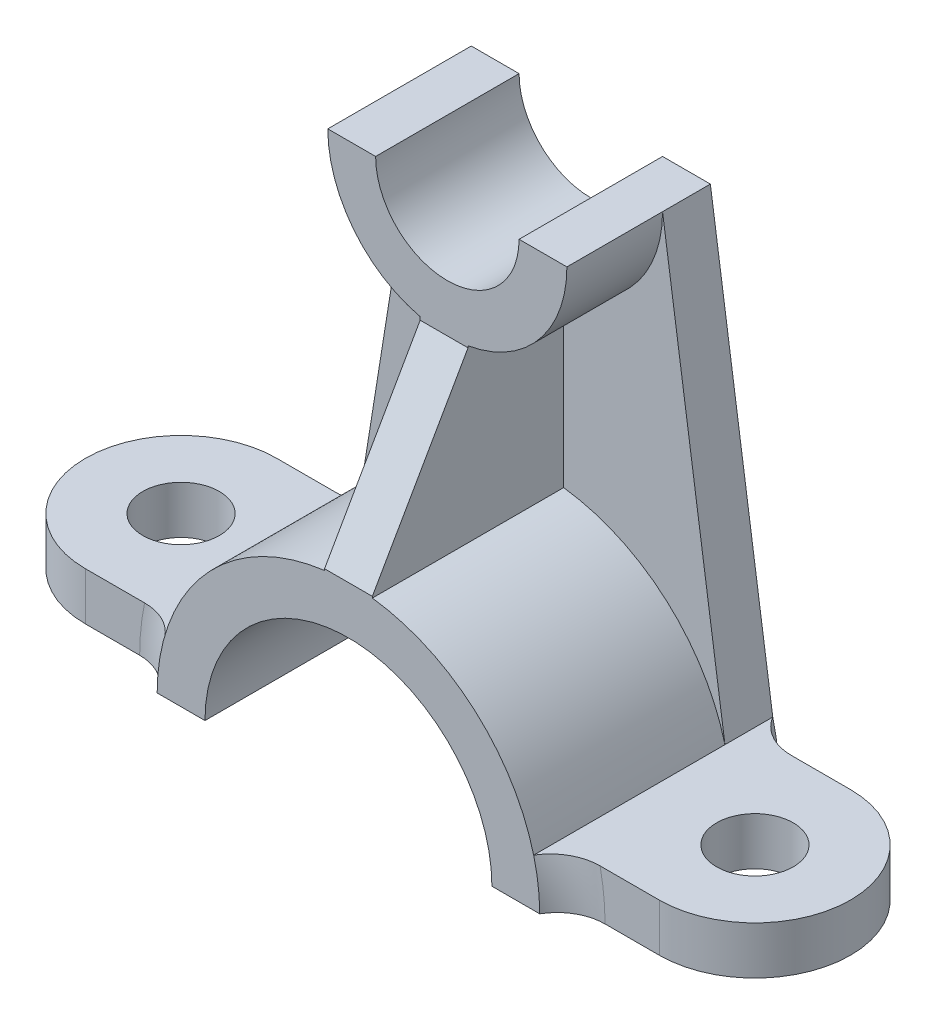
ISO-10303-21;
HEADER;
FILE_DESCRIPTION(('STEP AP214'),'2;1');
FILE_NAME('part.step','',(''),(''),'','','');
FILE_SCHEMA(('AUTOMOTIVE_DESIGN { 1 0 10303 214 1 1 1 1 }'));
ENDSEC;
DATA;
#1=APPLICATION_CONTEXT('core data for automotive mechanical design processes');
#2=APPLICATION_PROTOCOL_DEFINITION('international standard','automotive_design',2000,#1);
#3=PRODUCT_CONTEXT('',#1,'mechanical');
#4=PRODUCT('Part','Part','',(#3));
#5=PRODUCT_RELATED_PRODUCT_CATEGORY('part','',(#4));
#6=PRODUCT_DEFINITION_FORMATION('','',#4);
#7=PRODUCT_DEFINITION_CONTEXT('part definition',#1,'design');
#8=PRODUCT_DEFINITION('design','',#6,#7);
#9=PRODUCT_DEFINITION_SHAPE('','',#8);
#10=(LENGTH_UNIT() NAMED_UNIT(*) SI_UNIT(.MILLI.,.METRE.));
#11=(NAMED_UNIT(*) PLANE_ANGLE_UNIT() SI_UNIT($,.RADIAN.));
#12=(NAMED_UNIT(*) SI_UNIT($,.STERADIAN.) SOLID_ANGLE_UNIT());
#13=UNCERTAINTY_MEASURE_WITH_UNIT(LENGTH_MEASURE(1.E-05),#10,'distance_accuracy_value','');
#14=(GEOMETRIC_REPRESENTATION_CONTEXT(3) GLOBAL_UNCERTAINTY_ASSIGNED_CONTEXT((#13)) GLOBAL_UNIT_ASSIGNED_CONTEXT((#10,
#11,#12)) REPRESENTATION_CONTEXT('',''));
#15=CARTESIAN_POINT('',(0.,0.,0.));
#16=DIRECTION('',(0.,0.,1.));
#17=DIRECTION('',(1.,0.,0.));
#18=AXIS2_PLACEMENT_3D('',#15,#16,#17);
#19=CARTESIAN_POINT('',(0.,0.,25.));
#20=DIRECTION('',(0.,0.,-1.));
#21=DIRECTION('',(-1.,0.,0.));
#22=AXIS2_PLACEMENT_3D('',#19,#20,#21);
#23=CYLINDRICAL_SURFACE('',#22,40.);
#24=DIRECTION('',(0.,0.,-1.));
#25=VECTOR('',#24,1.);
#26=CARTESIAN_POINT('',(-5.,39.6862696659689,25.));
#27=LINE('',#26,#25);
#28=CARTESIAN_POINT('',(-5.,39.6862696659689,-15.));
#29=VERTEX_POINT('',#28);
#30=CARTESIAN_POINT('',(-5.,39.6862696659689,25.));
#31=VERTEX_POINT('',#30);
#32=EDGE_CURVE('E251',#29,#31,#27,.F.);
#33=ORIENTED_EDGE('',*,*,#32,.F.);
#34=CARTESIAN_POINT('',(0.,0.,-15.));
#35=DIRECTION('',(0.,0.,1.));
#36=DIRECTION('',(-1.,0.,0.));
#37=AXIS2_PLACEMENT_3D('',#34,#35,#36);
#38=CIRCLE('',#37,40.);
#39=CARTESIAN_POINT('',(-38.7298334620742,10.,-15.));
#40=VERTEX_POINT('',#39);
#41=EDGE_CURVE('E296',#29,#40,#38,.T.);
#42=ORIENTED_EDGE('',*,*,#41,.T.);
#43=DIRECTION('',(0.,0.,-1.));
#44=VECTOR('',#43,1.);
#45=CARTESIAN_POINT('',(-38.7298334620742,10.,25.));
#46=LINE('',#45,#44);
#47=CARTESIAN_POINT('',(-38.7298334620742,10.,25.));
#48=VERTEX_POINT('',#47);
#49=EDGE_CURVE('E399',#40,#48,#46,.F.);
#50=ORIENTED_EDGE('',*,*,#49,.T.);
#51=CARTESIAN_POINT('',(0.,0.,25.));
#52=DIRECTION('',(0.,0.,1.));
#53=DIRECTION('',(1.,0.,0.));
#54=AXIS2_PLACEMENT_3D('',#51,#52,#53);
#55=CIRCLE('',#54,40.);
#56=EDGE_CURVE('E372',#31,#48,#55,.T.);
#57=ORIENTED_EDGE('',*,*,#56,.F.);
#58=EDGE_LOOP('',(#33,#42,#50,#57));
#59=FACE_BOUND('',#58,.T.);
#60=ADVANCED_FACE('F39',(#59),#23,.T.);
#61=CARTESIAN_POINT('',(0.681025672357616,100.,-15.));
#62=DIRECTION('',(0.,0.,-1.));
#63=DIRECTION('',(-1.,0.,0.));
#64=AXIS2_PLACEMENT_3D('',#61,#62,#63);
#65=PLANE('',#64);
#66=DIRECTION('',(0.,-1.,0.));
#67=VECTOR('',#66,1.);
#68=CARTESIAN_POINT('',(-5.,100.,-15.));
#69=LINE('',#68,#67);
#70=CARTESIAN_POINT('',(-5.,75.6540363240636,-15.));
#71=VERTEX_POINT('',#70);
#72=EDGE_CURVE('E253',#71,#29,#69,.T.);
#73=ORIENTED_EDGE('',*,*,#72,.F.);
#74=CARTESIAN_POINT('',(0.681025672357616,100.,-15.));
#75=DIRECTION('',(0.,0.,1.));
#76=DIRECTION('',(-1.,0.,0.));
#77=AXIS2_PLACEMENT_3D('',#74,#75,#76);
#78=CIRCLE('',#77,25.);
#79=CARTESIAN_POINT('',(-24.3189743276424,100.,-15.));
#80=VERTEX_POINT('',#79);
#81=EDGE_CURVE('E291',#80,#71,#78,.T.);
#82=ORIENTED_EDGE('',*,*,#81,.F.);
#83=DIRECTION('',(0.158106665603804,0.987422038589198,0.));
#84=VECTOR('',#83,1.);
#85=CARTESIAN_POINT('',(-24.3189743276424,100.,-15.));
#86=LINE('',#85,#84);
#87=EDGE_CURVE('E303',#40,#80,#86,.T.);
#88=ORIENTED_EDGE('',*,*,#87,.F.);
#89=ORIENTED_EDGE('',*,*,#41,.F.);
#90=EDGE_LOOP('',(#73,#82,#88,#89));
#91=FACE_BOUND('',#90,.T.);
#92=ADVANCED_FACE('F475',(#91),#65,.F.);
#93=CARTESIAN_POINT('',(0.681025672357616,100.,5.));
#94=DIRECTION('',(0.,0.,-1.));
#95=DIRECTION('',(-1.,0.,0.));
#96=AXIS2_PLACEMENT_3D('',#93,#94,#95);
#97=CYLINDRICAL_SURFACE('',#96,25.);
#98=DIRECTION('',(0.,0.,-1.));
#99=VECTOR('',#98,1.);
#100=CARTESIAN_POINT('',(-5.,75.6540363240636,5.));
#101=LINE('',#100,#99);
#102=CARTESIAN_POINT('',(-5.,75.6540363240636,5.));
#103=VERTEX_POINT('',#102);
#104=EDGE_CURVE('E247',#103,#71,#101,.T.);
#105=ORIENTED_EDGE('',*,*,#104,.F.);
#106=CARTESIAN_POINT('',(0.681025672357616,100.,5.));
#107=DIRECTION('',(0.,0.,1.));
#108=DIRECTION('',(1.,0.,0.));
#109=AXIS2_PLACEMENT_3D('',#106,#107,#108);
#110=CIRCLE('',#109,25.);
#111=CARTESIAN_POINT('',(-24.3189743276424,100.,5.));
#112=VERTEX_POINT('',#111);
#113=EDGE_CURVE('E277',#112,#103,#110,.T.);
#114=ORIENTED_EDGE('',*,*,#113,.F.);
#115=DIRECTION('',(0.,0.,-1.));
#116=VECTOR('',#115,1.);
#117=CARTESIAN_POINT('',(-24.3189743276424,100.,5.));
#118=LINE('',#117,#116);
#119=EDGE_CURVE('E286',#112,#80,#118,.T.);
#120=ORIENTED_EDGE('',*,*,#119,.T.);
#121=ORIENTED_EDGE('',*,*,#81,.T.);
#122=EDGE_LOOP('',(#105,#114,#120,#121));
#123=FACE_BOUND('',#122,.T.);
#124=ADVANCED_FACE('F481',(#123),#97,.T.);
#125=CARTESIAN_POINT('',(38.7298334620742,10.,-15.));
#126=VERTEX_POINT('',#125);
#127=CARTESIAN_POINT('',(5.,39.6862696659689,-15.));
#128=VERTEX_POINT('',#127);
#129=EDGE_CURVE('E301',#126,#128,#38,.T.);
#130=ORIENTED_EDGE('',*,*,#129,.T.);
#131=DIRECTION('',(0.,0.,-1.));
#132=VECTOR('',#131,1.);
#133=CARTESIAN_POINT('',(5.,39.6862696659689,25.));
#134=LINE('',#133,#132);
#135=CARTESIAN_POINT('',(5.,39.6862696659689,25.));
#136=VERTEX_POINT('',#135);
#137=EDGE_CURVE('E261',#128,#136,#134,.F.);
#138=ORIENTED_EDGE('',*,*,#137,.T.);
#139=CARTESIAN_POINT('',(38.7298334620742,10.,25.));
#140=VERTEX_POINT('',#139);
#141=EDGE_CURVE('E234',#140,#136,#55,.T.);
#142=ORIENTED_EDGE('',*,*,#141,.F.);
#143=DIRECTION('',(0.,0.,-1.));
#144=VECTOR('',#143,1.);
#145=CARTESIAN_POINT('',(38.7298334620742,10.,25.));
#146=LINE('',#145,#144);
#147=EDGE_CURVE('E68',#126,#140,#146,.F.);
#148=ORIENTED_EDGE('',*,*,#147,.F.);
#149=EDGE_LOOP('',(#130,#138,#142,#148));
#150=FACE_BOUND('',#149,.T.);
#151=ADVANCED_FACE('F478',(#150),#23,.T.);
#152=CARTESIAN_POINT('',(-40.,0.,25.));
#153=DIRECTION('',(0.,1.,0.));
#154=DIRECTION('',(0.,0.,1.));
#155=AXIS2_PLACEMENT_3D('',#152,#153,#154);
#156=PLANE('',#155);
#157=CARTESIAN_POINT('',(-60.,0.,0.));
#158=DIRECTION('',(0.,1.,0.));
#159=DIRECTION('',(0.,0.,1.));
#160=AXIS2_PLACEMENT_3D('',#157,#158,#159);
#161=CIRCLE('',#160,8.);
#162=CARTESIAN_POINT('',(-60.,0.,8.));
#163=VERTEX_POINT('',#162);
#164=EDGE_CURVE('E314',#163,#163,#161,.T.);
#165=ORIENTED_EDGE('',*,*,#164,.T.);
#166=EDGE_LOOP('',(#165));
#167=FACE_BOUND('',#166,.T.);
#168=DIRECTION('',(1.,0.,0.));
#169=VECTOR('',#168,1.);
#170=CARTESIAN_POINT('',(-40.,0.,25.));
#171=LINE('',#170,#169);
#172=CARTESIAN_POINT('',(-40.,0.,25.));
#173=VERTEX_POINT('',#172);
#174=CARTESIAN_POINT('',(-30.,0.,25.));
#175=VERTEX_POINT('',#174);
#176=EDGE_CURVE('E373',#173,#175,#171,.T.);
#177=ORIENTED_EDGE('',*,*,#176,.F.);
#178=CARTESIAN_POINT('',(-48.6602540378444,0.,30.));
#179=DIRECTION('',(0.,1.,0.));
#180=DIRECTION('',(0.,0.,1.));
#181=AXIS2_PLACEMENT_3D('',#178,#179,#180);
#182=CIRCLE('',#181,10.);
#183=CARTESIAN_POINT('',(-48.6602540378444,0.,20.));
#184=VERTEX_POINT('',#183);
#185=EDGE_CURVE('E52',#173,#184,#182,.T.);
#186=ORIENTED_EDGE('',*,*,#185,.T.);
#187=DIRECTION('',(-1.,0.,0.));
#188=VECTOR('',#187,1.);
#189=CARTESIAN_POINT('',(-35.,0.,20.));
#190=LINE('',#189,#188);
#191=CARTESIAN_POINT('',(-60.,0.,20.));
#192=VERTEX_POINT('',#191);
#193=EDGE_CURVE('E341',#184,#192,#190,.T.);
#194=ORIENTED_EDGE('',*,*,#193,.T.);
#195=CARTESIAN_POINT('',(-60.,0.,0.));
#196=DIRECTION('',(0.,-1.,0.));
#197=DIRECTION('',(0.,0.,1.));
#198=AXIS2_PLACEMENT_3D('',#195,#196,#197);
#199=CIRCLE('',#198,20.);
#200=CARTESIAN_POINT('',(-60.,0.,-20.));
#201=VERTEX_POINT('',#200);
#202=EDGE_CURVE('E340',#192,#201,#199,.T.);
#203=ORIENTED_EDGE('',*,*,#202,.T.);
#204=DIRECTION('',(1.,0.,0.));
#205=VECTOR('',#204,1.);
#206=CARTESIAN_POINT('',(-35.,0.,-20.));
#207=LINE('',#206,#205);
#208=CARTESIAN_POINT('',(-48.6602540378444,0.,-20.));
#209=VERTEX_POINT('',#208);
#210=EDGE_CURVE('E331',#201,#209,#207,.T.);
#211=ORIENTED_EDGE('',*,*,#210,.T.);
#212=CARTESIAN_POINT('',(-48.6602540378444,0.,-30.));
#213=DIRECTION('',(0.,1.,0.));
#214=DIRECTION('',(0.,0.,1.));
#215=AXIS2_PLACEMENT_3D('',#212,#213,#214);
#216=CIRCLE('',#215,10.);
#217=CARTESIAN_POINT('',(-40.,0.,-25.));
#218=VERTEX_POINT('',#217);
#219=EDGE_CURVE('E420',#209,#218,#216,.T.);
#220=ORIENTED_EDGE('',*,*,#219,.T.);
#221=DIRECTION('',(1.,0.,0.));
#222=VECTOR('',#221,1.);
#223=CARTESIAN_POINT('',(-40.,0.,-25.));
#224=LINE('',#223,#222);
#225=CARTESIAN_POINT('',(-30.,0.,-25.));
#226=VERTEX_POINT('',#225);
#227=EDGE_CURVE('E384',#218,#226,#224,.T.);
#228=ORIENTED_EDGE('',*,*,#227,.T.);
#229=DIRECTION('',(0.,0.,-1.));
#230=VECTOR('',#229,1.);
#231=CARTESIAN_POINT('',(-30.,0.,25.));
#232=LINE('',#231,#230);
#233=EDGE_CURVE('E391',#175,#226,#232,.T.);
#234=ORIENTED_EDGE('',*,*,#233,.F.);
#235=EDGE_LOOP('',(#177,#186,#194,#203,#211,#220,#228,#234));
#236=FACE_BOUND('',#235,.T.);
#237=ADVANCED_FACE('F488',(#167,#236),#156,.F.);
#238=CARTESIAN_POINT('',(0.,0.,25.));
#239=DIRECTION('',(0.,0.,-1.));
#240=DIRECTION('',(-1.,0.,0.));
#241=AXIS2_PLACEMENT_3D('',#238,#239,#240);
#242=CYLINDRICAL_SURFACE('',#241,30.);
#243=DIRECTION('',(0.,0.,-1.));
#244=VECTOR('',#243,1.);
#245=CARTESIAN_POINT('',(30.,0.,25.));
#246=LINE('',#245,#244);
#247=CARTESIAN_POINT('',(30.,0.,25.));
#248=VERTEX_POINT('',#247);
#249=CARTESIAN_POINT('',(30.,0.,-25.));
#250=VERTEX_POINT('',#249);
#251=EDGE_CURVE('E381',#248,#250,#246,.T.);
#252=ORIENTED_EDGE('',*,*,#251,.F.);
#253=CARTESIAN_POINT('',(0.,0.,25.));
#254=DIRECTION('',(0.,0.,-1.));
#255=DIRECTION('',(1.,0.,0.));
#256=AXIS2_PLACEMENT_3D('',#253,#254,#255);
#257=CIRCLE('',#256,30.);
#258=EDGE_CURVE('E376',#175,#248,#257,.T.);
#259=ORIENTED_EDGE('',*,*,#258,.F.);
#260=ORIENTED_EDGE('',*,*,#233,.T.);
#261=CARTESIAN_POINT('',(0.,0.,-25.));
#262=DIRECTION('',(0.,0.,-1.));
#263=DIRECTION('',(1.,0.,0.));
#264=AXIS2_PLACEMENT_3D('',#261,#262,#263);
#265=CIRCLE('',#264,30.);
#266=EDGE_CURVE('E390',#226,#250,#265,.T.);
#267=ORIENTED_EDGE('',*,*,#266,.T.);
#268=EDGE_LOOP('',(#252,#259,#260,#267));
#269=FACE_BOUND('',#268,.T.);
#270=ADVANCED_FACE('F493',(#269),#242,.F.);
#271=CARTESIAN_POINT('',(30.,0.,25.));
#272=DIRECTION('',(0.,1.,0.));
#273=DIRECTION('',(0.,0.,1.));
#274=AXIS2_PLACEMENT_3D('',#271,#272,#273);
#275=PLANE('',#274);
#276=CARTESIAN_POINT('',(60.,0.,0.));
#277=DIRECTION('',(0.,1.,0.));
#278=DIRECTION('',(0.,0.,1.));
#279=AXIS2_PLACEMENT_3D('',#276,#277,#278);
#280=CIRCLE('',#279,8.00000000000001);
#281=CARTESIAN_POINT('',(60.,0.,8.00000000000001));
#282=VERTEX_POINT('',#281);
#283=EDGE_CURVE('E320',#282,#282,#280,.T.);
#284=ORIENTED_EDGE('',*,*,#283,.T.);
#285=EDGE_LOOP('',(#284));
#286=FACE_BOUND('',#285,.T.);
#287=DIRECTION('',(1.,0.,0.));
#288=VECTOR('',#287,1.);
#289=CARTESIAN_POINT('',(30.,0.,-25.));
#290=LINE('',#289,#288);
#291=CARTESIAN_POINT('',(40.,0.,-25.));
#292=VERTEX_POINT('',#291);
#293=EDGE_CURVE('E386',#250,#292,#290,.T.);
#294=ORIENTED_EDGE('',*,*,#293,.T.);
#295=CARTESIAN_POINT('',(48.6602540378444,0.,-30.));
#296=DIRECTION('',(0.,1.,0.));
#297=DIRECTION('',(0.,0.,1.));
#298=AXIS2_PLACEMENT_3D('',#295,#296,#297);
#299=CIRCLE('',#298,10.);
#300=CARTESIAN_POINT('',(48.6602540378444,0.,-20.));
#301=VERTEX_POINT('',#300);
#302=EDGE_CURVE('E576',#292,#301,#299,.T.);
#303=ORIENTED_EDGE('',*,*,#302,.T.);
#304=DIRECTION('',(1.,0.,0.));
#305=VECTOR('',#304,1.);
#306=CARTESIAN_POINT('',(35.,0.,-20.));
#307=LINE('',#306,#305);
#308=CARTESIAN_POINT('',(60.,0.,-20.));
#309=VERTEX_POINT('',#308);
#310=EDGE_CURVE('E343',#301,#309,#307,.T.);
#311=ORIENTED_EDGE('',*,*,#310,.T.);
#312=CARTESIAN_POINT('',(60.,0.,0.));
#313=DIRECTION('',(0.,-1.,0.));
#314=DIRECTION('',(0.,0.,-1.));
#315=AXIS2_PLACEMENT_3D('',#312,#313,#314);
#316=CIRCLE('',#315,20.);
#317=CARTESIAN_POINT('',(60.,0.,20.));
#318=VERTEX_POINT('',#317);
#319=EDGE_CURVE('E363',#309,#318,#316,.T.);
#320=ORIENTED_EDGE('',*,*,#319,.T.);
#321=DIRECTION('',(-1.,0.,0.));
#322=VECTOR('',#321,1.);
#323=CARTESIAN_POINT('',(35.,0.,20.));
#324=LINE('',#323,#322);
#325=CARTESIAN_POINT('',(48.6602540378444,0.,20.));
#326=VERTEX_POINT('',#325);
#327=EDGE_CURVE('E353',#318,#326,#324,.T.);
#328=ORIENTED_EDGE('',*,*,#327,.T.);
#329=CARTESIAN_POINT('',(48.6602540378444,0.,30.));
#330=DIRECTION('',(0.,1.,0.));
#331=DIRECTION('',(0.,0.,1.));
#332=AXIS2_PLACEMENT_3D('',#329,#330,#331);
#333=CIRCLE('',#332,10.);
#334=CARTESIAN_POINT('',(40.,0.,25.));
#335=VERTEX_POINT('',#334);
#336=EDGE_CURVE('E460',#326,#335,#333,.T.);
#337=ORIENTED_EDGE('',*,*,#336,.T.);
#338=DIRECTION('',(1.,0.,0.));
#339=VECTOR('',#338,1.);
#340=CARTESIAN_POINT('',(30.,0.,25.));
#341=LINE('',#340,#339);
#342=EDGE_CURVE('E378',#248,#335,#341,.T.);
#343=ORIENTED_EDGE('',*,*,#342,.F.);
#344=ORIENTED_EDGE('',*,*,#251,.T.);
#345=EDGE_LOOP('',(#294,#303,#311,#320,#328,#337,#343,#344));
#346=FACE_BOUND('',#345,.T.);
#347=ADVANCED_FACE('F804',(#286,#346),#275,.F.);
#348=CARTESIAN_POINT('',(0.,0.,25.));
#349=DIRECTION('',(0.,0.,1.));
#350=DIRECTION('',(1.,0.,0.));
#351=AXIS2_PLACEMENT_3D('',#348,#349,#350);
#352=PLANE('',#351);
#353=ORIENTED_EDGE('',*,*,#141,.T.);
#354=DIRECTION('',(0.,1.,0.));
#355=VECTOR('',#354,1.);
#356=CARTESIAN_POINT('',(5.,50.,25.));
#357=LINE('',#356,#355);
#358=CARTESIAN_POINT('',(5.,40.,25.));
#359=VERTEX_POINT('',#358);
#360=EDGE_CURVE('E226',#136,#359,#357,.T.);
#361=ORIENTED_EDGE('',*,*,#360,.T.);
#362=DIRECTION('',(1.,0.,0.));
#363=VECTOR('',#362,1.);
#364=CARTESIAN_POINT('',(0.,40.,25.));
#365=LINE('',#364,#363);
#366=CARTESIAN_POINT('',(-5.,40.,25.));
#367=VERTEX_POINT('',#366);
#368=EDGE_CURVE('E219',#367,#359,#365,.T.);
#369=ORIENTED_EDGE('',*,*,#368,.F.);
#370=DIRECTION('',(0.,1.,0.));
#371=VECTOR('',#370,1.);
#372=CARTESIAN_POINT('',(-5.,50.,25.));
#373=LINE('',#372,#371);
#374=EDGE_CURVE('E242',#31,#367,#373,.T.);
#375=ORIENTED_EDGE('',*,*,#374,.F.);
#376=ORIENTED_EDGE('',*,*,#56,.T.);
#377=EDGE_CURVE('E395',#48,#173,#55,.T.);
#378=ORIENTED_EDGE('',*,*,#377,.T.);
#379=ORIENTED_EDGE('',*,*,#176,.T.);
#380=ORIENTED_EDGE('',*,*,#258,.T.);
#381=ORIENTED_EDGE('',*,*,#342,.T.);
#382=EDGE_CURVE('E371',#335,#140,#55,.T.);
#383=ORIENTED_EDGE('',*,*,#382,.T.);
#384=EDGE_LOOP('',(#353,#361,#369,#375,#376,#378,#379,#380,#381,#383));
#385=FACE_BOUND('',#384,.T.);
#386=ADVANCED_FACE('F233',(#385),#352,.T.);
#387=CARTESIAN_POINT('',(0.,0.,-25.));
#388=DIRECTION('',(0.,0.,1.));
#389=DIRECTION('',(1.,0.,0.));
#390=AXIS2_PLACEMENT_3D('',#387,#388,#389);
#391=PLANE('',#390);
#392=ORIENTED_EDGE('',*,*,#293,.F.);
#393=ORIENTED_EDGE('',*,*,#266,.F.);
#394=ORIENTED_EDGE('',*,*,#227,.F.);
#395=CARTESIAN_POINT('',(0.,0.,-25.));
#396=DIRECTION('',(0.,0.,1.));
#397=DIRECTION('',(1.,0.,0.));
#398=AXIS2_PLACEMENT_3D('',#395,#396,#397);
#399=CIRCLE('',#398,40.);
#400=CARTESIAN_POINT('',(-38.7298334620742,10.,-25.));
#401=VERTEX_POINT('',#400);
#402=EDGE_CURVE('E366',#401,#218,#399,.T.);
#403=ORIENTED_EDGE('',*,*,#402,.F.);
#404=DIRECTION('',(0.158106665603804,0.987422038589198,0.));
#405=VECTOR('',#404,1.);
#406=CARTESIAN_POINT('',(-24.3189743276424,100.,-25.));
#407=LINE('',#406,#405);
#408=CARTESIAN_POINT('',(-24.3189743276424,100.,-25.));
#409=VERTEX_POINT('',#408);
#410=EDGE_CURVE('E310',#401,#409,#407,.T.);
#411=ORIENTED_EDGE('',*,*,#410,.T.);
#412=DIRECTION('',(-1.,0.,0.));
#413=VECTOR('',#412,1.);
#414=CARTESIAN_POINT('',(-24.3189743276424,100.,-25.));
#415=LINE('',#414,#413);
#416=CARTESIAN_POINT('',(-14.3189743276424,100.,-25.));
#417=VERTEX_POINT('',#416);
#418=EDGE_CURVE('E264',#417,#409,#415,.T.);
#419=ORIENTED_EDGE('',*,*,#418,.F.);
#420=CARTESIAN_POINT('',(0.681025672357616,100.,-25.));
#421=DIRECTION('',(0.,0.,-1.));
#422=DIRECTION('',(1.,0.,0.));
#423=AXIS2_PLACEMENT_3D('',#420,#421,#422);
#424=CIRCLE('',#423,15.);
#425=CARTESIAN_POINT('',(15.6810256723576,100.,-25.));
#426=VERTEX_POINT('',#425);
#427=EDGE_CURVE('E263',#426,#417,#424,.T.);
#428=ORIENTED_EDGE('',*,*,#427,.F.);
#429=DIRECTION('',(-1.,0.,0.));
#430=VECTOR('',#429,1.);
#431=CARTESIAN_POINT('',(15.6810256723576,100.,-25.));
#432=LINE('',#431,#430);
#433=CARTESIAN_POINT('',(25.6810256723576,100.,-25.));
#434=VERTEX_POINT('',#433);
#435=EDGE_CURVE('E268',#434,#426,#432,.T.);
#436=ORIENTED_EDGE('',*,*,#435,.F.);
#437=DIRECTION('',(0.143486470703755,-0.989652278694381,0.));
#438=VECTOR('',#437,1.);
#439=CARTESIAN_POINT('',(25.6810256723576,100.,-25.));
#440=LINE('',#439,#438);
#441=CARTESIAN_POINT('',(38.7298334620742,10.,-25.));
#442=VERTEX_POINT('',#441);
#443=EDGE_CURVE('E295',#434,#442,#440,.T.);
#444=ORIENTED_EDGE('',*,*,#443,.T.);
#445=EDGE_CURVE('E385',#292,#442,#399,.T.);
#446=ORIENTED_EDGE('',*,*,#445,.F.);
#447=EDGE_LOOP('',(#392,#393,#394,#403,#411,#419,#428,#436,#444,#446));
#448=FACE_BOUND('',#447,.T.);
#449=ADVANCED_FACE('F439',(#448),#391,.F.);
#450=CARTESIAN_POINT('',(60.,10.,0.));
#451=DIRECTION('',(0.,-1.,0.));
#452=DIRECTION('',(0.,0.,-1.));
#453=AXIS2_PLACEMENT_3D('',#450,#451,#452);
#454=PLANE('',#453);
#455=CARTESIAN_POINT('',(60.,10.,0.));
#456=DIRECTION('',(0.,1.,0.));
#457=DIRECTION('',(0.,0.,1.));
#458=AXIS2_PLACEMENT_3D('',#455,#456,#457);
#459=CIRCLE('',#458,8.00000000000001);
#460=CARTESIAN_POINT('',(60.,10.,8.00000000000001));
#461=VERTEX_POINT('',#460);
#462=EDGE_CURVE('E321',#461,#461,#459,.T.);
#463=ORIENTED_EDGE('',*,*,#462,.F.);
#464=EDGE_LOOP('',(#463));
#465=FACE_BOUND('',#464,.T.);
#466=DIRECTION('',(1.,0.,0.));
#467=VECTOR('',#466,1.);
#468=CARTESIAN_POINT('',(35.,10.,-20.));
#469=LINE('',#468,#467);
#470=CARTESIAN_POINT('',(47.6216371309046,10.,-20.));
#471=VERTEX_POINT('',#470);
#472=CARTESIAN_POINT('',(60.,10.,-20.));
#473=VERTEX_POINT('',#472);
#474=EDGE_CURVE('E348',#471,#473,#469,.T.);
#475=ORIENTED_EDGE('',*,*,#474,.F.);
#476=CARTESIAN_POINT('',(47.6216371309046,10.,-20.));
#477=CARTESIAN_POINT('',(47.3275635647128,10.,-19.9999725811996));
#478=CARTESIAN_POINT('',(47.0334977113731,10.,-20.01242289388));
#479=CARTESIAN_POINT('',(46.4474700390628,10.,-20.0620205132552));
#480=CARTESIAN_POINT('',(46.155508114054,10.,-20.0991665663559));
#481=CARTESIAN_POINT('',(45.575958192143,10.,-20.1978612196002));
#482=CARTESIAN_POINT('',(45.2883671585936,10.,-20.2593919906349));
#483=CARTESIAN_POINT('',(44.7193773078864,10.,-20.4064113995505));
#484=CARTESIAN_POINT('',(44.4379784487489,10.,-20.4918998749561));
#485=CARTESIAN_POINT('',(43.883221966373,10.,-20.686310813259));
#486=CARTESIAN_POINT('',(43.6098688058399,10.,-20.7952460129183));
#487=CARTESIAN_POINT('',(43.0732082863903,10.,-21.0358552040146));
#488=CARTESIAN_POINT('',(42.809905561898,10.,-21.1675395344293));
#489=CARTESIAN_POINT('',(42.295507191387,10.,-21.4526919145932));
#490=CARTESIAN_POINT('',(42.0444066771186,10.,-21.6061511795191));
#491=CARTESIAN_POINT('',(41.5562899807496,10.,-21.9338095330143));
#492=CARTESIAN_POINT('',(41.319267310127,10.,-22.1079989540299));
#493=CARTESIAN_POINT('',(40.8558274604119,10.,-22.4801785915545));
#494=CARTESIAN_POINT('',(40.6297696026495,10.,-22.6786166712502));
#495=CARTESIAN_POINT('',(40.1960204197636,10.,-23.0946419762966));
#496=CARTESIAN_POINT('',(39.9883288915656,10.,-23.3122289898663));
#497=CARTESIAN_POINT('',(39.5925441910588,10.,-23.7656411050683));
#498=CARTESIAN_POINT('',(39.4045075329251,10.,-24.0015155760535));
#499=CARTESIAN_POINT('',(39.0503222140867,10.,-24.4892347345405));
#500=CARTESIAN_POINT('',(38.8841782881545,10.,-24.7410828592982));
#501=CARTESIAN_POINT('',(38.7298334620742,10.,-25.));
#502=B_SPLINE_CURVE_WITH_KNOTS('',3,(#476,#477,#478,#479,#480,#481,#482,#483,#484,#485,#486,
#487,#488,#489,#490,#491,#492,#493,#494,#495,#496,#497,#498,#499,#500,#501),.UNSPECIFIED.,.F.,
.F.,(4,2,2,2,2,2,2,2,2,2,2,2,4),(0.,0.881946521958427,1.76384827836067,2.64510641038706,
3.52635856607926,4.40809065046293,5.2902245219269,6.17200351413211,7.05337288641838,
7.95460227176324,8.85582169106561,9.75956497952399,10.6635034021589),.UNSPECIFIED.);
#503=EDGE_CURVE('E443',#471,#442,#502,.T.);
#504=ORIENTED_EDGE('',*,*,#503,.T.);
#505=EDGE_CURVE('E398',#442,#126,#146,.F.);
#506=ORIENTED_EDGE('',*,*,#505,.T.);
#507=ORIENTED_EDGE('',*,*,#147,.T.);
#508=CARTESIAN_POINT('',(38.7298334620742,10.,25.));
#509=CARTESIAN_POINT('',(38.8768130946296,10.,24.7534474368264));
#510=CARTESIAN_POINT('',(39.0344881880788,10.,24.5132998701854));
#511=CARTESIAN_POINT('',(39.3697661682135,10.,24.0474146522238));
#512=CARTESIAN_POINT('',(39.5473649268116,10.,23.821674031005));
#513=CARTESIAN_POINT('',(39.9206019875073,10.,23.3866670743957));
#514=CARTESIAN_POINT('',(40.1161920586549,10.,23.1773593289555));
#515=CARTESIAN_POINT('',(40.5242729292274,10.,22.7759168816667));
#516=CARTESIAN_POINT('',(40.7367642892412,10.,22.5837827498889));
#517=CARTESIAN_POINT('',(41.1769775394081,10.,22.2179742792945));
#518=CARTESIAN_POINT('',(41.4046951784532,10.,22.0442948227889));
#519=CARTESIAN_POINT('',(41.8738510913466,10.,21.7163510300474));
#520=CARTESIAN_POINT('',(42.1152953822557,10.,21.5620953049238));
#521=CARTESIAN_POINT('',(42.6102602764297,10.,21.2739519840888));
#522=CARTESIAN_POINT('',(42.8637887877046,10.,21.1400779734591));
#523=CARTESIAN_POINT('',(43.380892368368,10.,20.8937049439873));
#524=CARTESIAN_POINT('',(43.6444633858867,10.,20.7811974117538));
#525=CARTESIAN_POINT('',(44.2074399218215,10.,20.5677750708857));
#526=CARTESIAN_POINT('',(44.507748060584,10.,20.4692329711595));
#527=CARTESIAN_POINT('',(45.1160624466181,10.,20.2996699213064));
#528=CARTESIAN_POINT('',(45.4240695595761,10.,20.2286520810099));
#529=CARTESIAN_POINT('',(46.0457021235101,10.,20.1146504402653));
#530=CARTESIAN_POINT('',(46.3593351985563,10.,20.0717081872946));
#531=CARTESIAN_POINT('',(46.9891881697605,10.,20.0143649506646));
#532=CARTESIAN_POINT('',(47.3054079836948,10.,19.9999630633169));
#533=CARTESIAN_POINT('',(47.6216371309046,10.,20.));
#534=B_SPLINE_CURVE_WITH_KNOTS('',3,(#508,#509,#510,#511,#512,#513,#514,#515,#516,#517,#518,
#519,#520,#521,#522,#523,#524,#525,#526,#527,#528,#529,#530,#531,#532,#533),.UNSPECIFIED.,.F.,
.F.,(4,2,2,2,2,2,2,2,2,2,2,2,4),(0.,0.860812450935914,1.72144687394709,2.57983785811531,
3.43825732563233,4.29643811907591,5.15499803978743,6.01412773684447,6.87291439544276,
7.81978670139646,8.76676595862135,9.71514344396407,10.663490899854),.UNSPECIFIED.);
#535=CARTESIAN_POINT('',(47.6216371309046,10.,20.));
#536=VERTEX_POINT('',#535);
#537=EDGE_CURVE('E451',#140,#536,#534,.T.);
#538=ORIENTED_EDGE('',*,*,#537,.T.);
#539=DIRECTION('',(-1.,0.,0.));
#540=VECTOR('',#539,1.);
#541=CARTESIAN_POINT('',(35.,10.,20.));
#542=LINE('',#541,#540);
#543=CARTESIAN_POINT('',(60.,10.,20.));
#544=VERTEX_POINT('',#543);
#545=EDGE_CURVE('E356',#544,#536,#542,.T.);
#546=ORIENTED_EDGE('',*,*,#545,.F.);
#547=CARTESIAN_POINT('',(60.,10.,0.));
#548=DIRECTION('',(0.,-1.,0.));
#549=DIRECTION('',(0.,0.,-1.));
#550=AXIS2_PLACEMENT_3D('',#547,#548,#549);
#551=CIRCLE('',#550,20.);
#552=EDGE_CURVE('E355',#473,#544,#551,.T.);
#553=ORIENTED_EDGE('',*,*,#552,.F.);
#554=EDGE_LOOP('',(#475,#504,#506,#507,#538,#546,#553));
#555=FACE_BOUND('',#554,.T.);
#556=ADVANCED_FACE('F432',(#465,#555),#454,.F.);
#557=CARTESIAN_POINT('',(35.,10.,20.));
#558=DIRECTION('',(0.,0.,1.));
#559=DIRECTION('',(1.,0.,0.));
#560=AXIS2_PLACEMENT_3D('',#557,#558,#559);
#561=PLANE('',#560);
#562=ORIENTED_EDGE('',*,*,#545,.T.);
#563=CARTESIAN_POINT('',(0.,0.,20.));
#564=DIRECTION('',(0.,0.,1.));
#565=DIRECTION('',(1.,0.,0.));
#566=AXIS2_PLACEMENT_3D('',#563,#564,#565);
#567=CIRCLE('',#566,48.6602540378444);
#568=EDGE_CURVE('E408',#536,#326,#567,.F.);
#569=ORIENTED_EDGE('',*,*,#568,.T.);
#570=ORIENTED_EDGE('',*,*,#327,.F.);
#571=DIRECTION('',(0.,-1.,0.));
#572=VECTOR('',#571,1.);
#573=CARTESIAN_POINT('',(60.,10.,20.));
#574=LINE('',#573,#572);
#575=EDGE_CURVE('E368',#544,#318,#574,.T.);
#576=ORIENTED_EDGE('',*,*,#575,.F.);
#577=EDGE_LOOP('',(#562,#569,#570,#576));
#578=FACE_BOUND('',#577,.T.);
#579=ADVANCED_FACE('F438',(#578),#561,.T.);
#580=CARTESIAN_POINT('',(35.,10.,-20.));
#581=DIRECTION('',(0.,0.,-1.));
#582=DIRECTION('',(-1.,0.,0.));
#583=AXIS2_PLACEMENT_3D('',#580,#581,#582);
#584=PLANE('',#583);
#585=ORIENTED_EDGE('',*,*,#310,.F.);
#586=CARTESIAN_POINT('',(0.,0.,-20.));
#587=DIRECTION('',(0.,0.,-1.));
#588=DIRECTION('',(-1.,0.,0.));
#589=AXIS2_PLACEMENT_3D('',#586,#587,#588);
#590=CIRCLE('',#589,48.6602540378444);
#591=EDGE_CURVE('E407',#301,#471,#590,.F.);
#592=ORIENTED_EDGE('',*,*,#591,.T.);
#593=ORIENTED_EDGE('',*,*,#474,.T.);
#594=DIRECTION('',(0.,-1.,0.));
#595=VECTOR('',#594,1.);
#596=CARTESIAN_POINT('',(60.,10.,-20.));
#597=LINE('',#596,#595);
#598=EDGE_CURVE('E357',#473,#309,#597,.T.);
#599=ORIENTED_EDGE('',*,*,#598,.T.);
#600=EDGE_LOOP('',(#585,#592,#593,#599));
#601=FACE_BOUND('',#600,.T.);
#602=ADVANCED_FACE('F772',(#601),#584,.T.);
#603=CARTESIAN_POINT('',(60.,10.,0.));
#604=DIRECTION('',(0.,-1.,0.));
#605=DIRECTION('',(0.,0.,-1.));
#606=AXIS2_PLACEMENT_3D('',#603,#604,#605);
#607=CYLINDRICAL_SURFACE('',#606,20.);
#608=ORIENTED_EDGE('',*,*,#319,.F.);
#609=ORIENTED_EDGE('',*,*,#598,.F.);
#610=ORIENTED_EDGE('',*,*,#552,.T.);
#611=ORIENTED_EDGE('',*,*,#575,.T.);
#612=EDGE_LOOP('',(#608,#609,#610,#611));
#613=FACE_BOUND('',#612,.T.);
#614=ADVANCED_FACE('F431',(#613),#607,.T.);
#615=CARTESIAN_POINT('',(-60.,10.,0.));
#616=DIRECTION('',(0.,1.,0.));
#617=DIRECTION('',(0.,0.,1.));
#618=AXIS2_PLACEMENT_3D('',#615,#616,#617);
#619=PLANE('',#618);
#620=CARTESIAN_POINT('',(-60.,10.,0.));
#621=DIRECTION('',(0.,1.,0.));
#622=DIRECTION('',(0.,0.,1.));
#623=AXIS2_PLACEMENT_3D('',#620,#621,#622);
#624=CIRCLE('',#623,8.);
#625=CARTESIAN_POINT('',(-60.,10.,8.));
#626=VERTEX_POINT('',#625);
#627=EDGE_CURVE('E322',#626,#626,#624,.T.);
#628=ORIENTED_EDGE('',*,*,#627,.F.);
#629=EDGE_LOOP('',(#628));
#630=FACE_BOUND('',#629,.T.);
#631=EDGE_CURVE('E402',#401,#40,#46,.F.);
#632=ORIENTED_EDGE('',*,*,#631,.F.);
#633=CARTESIAN_POINT('',(-38.7298334620742,10.,-25.));
#634=CARTESIAN_POINT('',(-38.8768130946296,10.,-24.7534474368264));
#635=CARTESIAN_POINT('',(-39.0344881880788,10.,-24.5132998701854));
#636=CARTESIAN_POINT('',(-39.3697661682135,10.,-24.0474146522238));
#637=CARTESIAN_POINT('',(-39.5473649268116,10.,-23.821674031005));
#638=CARTESIAN_POINT('',(-39.9206019875073,10.,-23.3866670743957));
#639=CARTESIAN_POINT('',(-40.1161920586549,10.,-23.1773593289555));
#640=CARTESIAN_POINT('',(-40.5242729292274,10.,-22.7759168816667));
#641=CARTESIAN_POINT('',(-40.7367642892412,10.,-22.5837827498889));
#642=CARTESIAN_POINT('',(-41.1769775394081,10.,-22.2179742792945));
#643=CARTESIAN_POINT('',(-41.4046951784532,10.,-22.0442948227889));
#644=CARTESIAN_POINT('',(-41.8738510913466,10.,-21.7163510300474));
#645=CARTESIAN_POINT('',(-42.1152953822557,10.,-21.5620953049238));
#646=CARTESIAN_POINT('',(-42.6102602764297,10.,-21.2739519840888));
#647=CARTESIAN_POINT('',(-42.8637887877046,10.,-21.1400779734591));
#648=CARTESIAN_POINT('',(-43.380892368368,10.,-20.8937049439873));
#649=CARTESIAN_POINT('',(-43.6444633858867,10.,-20.7811974117538));
#650=CARTESIAN_POINT('',(-44.2074399218215,10.,-20.5677750708857));
#651=CARTESIAN_POINT('',(-44.507748060584,10.,-20.4692329711595));
#652=CARTESIAN_POINT('',(-45.1160624466181,10.,-20.2996699213064));
#653=CARTESIAN_POINT('',(-45.4240695595761,10.,-20.2286520810099));
#654=CARTESIAN_POINT('',(-46.0457021235101,10.,-20.1146504402653));
#655=CARTESIAN_POINT('',(-46.3593351985563,10.,-20.0717081872946));
#656=CARTESIAN_POINT('',(-46.9891881697605,10.,-20.0143649506646));
#657=CARTESIAN_POINT('',(-47.3054079836948,10.,-19.9999630633169));
#658=CARTESIAN_POINT('',(-47.6216371309046,10.,-20.));
#659=B_SPLINE_CURVE_WITH_KNOTS('',3,(#633,#634,#635,#636,#637,#638,#639,#640,#641,#642,#643,
#644,#645,#646,#647,#648,#649,#650,#651,#652,#653,#654,#655,#656,#657,#658),.UNSPECIFIED.,.F.,
.F.,(4,2,2,2,2,2,2,2,2,2,2,2,4),(0.,0.860812450935914,1.72144687394709,2.57983785811531,
3.43825732563233,4.29643811907591,5.15499803978743,6.01412773684447,6.87291439544276,
7.81978670139646,8.76676595862135,9.71514344396407,10.663490899854),.UNSPECIFIED.);
#660=CARTESIAN_POINT('',(-47.6216371309046,10.,-20.));
#661=VERTEX_POINT('',#660);
#662=EDGE_CURVE('E415',#401,#661,#659,.T.);
#663=ORIENTED_EDGE('',*,*,#662,.T.);
#664=DIRECTION('',(1.,0.,0.));
#665=VECTOR('',#664,1.);
#666=CARTESIAN_POINT('',(-35.,10.,-20.));
#667=LINE('',#666,#665);
#668=CARTESIAN_POINT('',(-60.,10.,-20.));
#669=VERTEX_POINT('',#668);
#670=EDGE_CURVE('E335',#669,#661,#667,.T.);
#671=ORIENTED_EDGE('',*,*,#670,.F.);
#672=CARTESIAN_POINT('',(-60.,10.,0.));
#673=DIRECTION('',(0.,-1.,0.));
#674=DIRECTION('',(0.,0.,1.));
#675=AXIS2_PLACEMENT_3D('',#672,#673,#674);
#676=CIRCLE('',#675,20.);
#677=CARTESIAN_POINT('',(-60.,10.,20.));
#678=VERTEX_POINT('',#677);
#679=EDGE_CURVE('E347',#678,#669,#676,.T.);
#680=ORIENTED_EDGE('',*,*,#679,.F.);
#681=DIRECTION('',(-1.,0.,0.));
#682=VECTOR('',#681,1.);
#683=CARTESIAN_POINT('',(-35.,10.,20.));
#684=LINE('',#683,#682);
#685=CARTESIAN_POINT('',(-47.6216371309046,10.,20.));
#686=VERTEX_POINT('',#685);
#687=EDGE_CURVE('E338',#686,#678,#684,.T.);
#688=ORIENTED_EDGE('',*,*,#687,.F.);
#689=CARTESIAN_POINT('',(-47.6216371309046,10.,20.));
#690=CARTESIAN_POINT('',(-47.3275635647128,10.,19.9999725811996));
#691=CARTESIAN_POINT('',(-47.0334977113731,10.,20.01242289388));
#692=CARTESIAN_POINT('',(-46.4474700390628,10.,20.0620205132552));
#693=CARTESIAN_POINT('',(-46.155508114054,10.,20.0991665663559));
#694=CARTESIAN_POINT('',(-45.575958192143,10.,20.1978612196002));
#695=CARTESIAN_POINT('',(-45.2883671585936,10.,20.2593919906349));
#696=CARTESIAN_POINT('',(-44.7193773078864,10.,20.4064113995505));
#697=CARTESIAN_POINT('',(-44.4379784487489,10.,20.4918998749561));
#698=CARTESIAN_POINT('',(-43.883221966373,10.,20.686310813259));
#699=CARTESIAN_POINT('',(-43.6098688058399,10.,20.7952460129183));
#700=CARTESIAN_POINT('',(-43.0732082863903,10.,21.0358552040146));
#701=CARTESIAN_POINT('',(-42.809905561898,10.,21.1675395344293));
#702=CARTESIAN_POINT('',(-42.295507191387,10.,21.4526919145932));
#703=CARTESIAN_POINT('',(-42.0444066771186,10.,21.6061511795191));
#704=CARTESIAN_POINT('',(-41.5562899807496,10.,21.9338095330143));
#705=CARTESIAN_POINT('',(-41.319267310127,10.,22.1079989540299));
#706=CARTESIAN_POINT('',(-40.8558274604119,10.,22.4801785915545));
#707=CARTESIAN_POINT('',(-40.6297696026495,10.,22.6786166712502));
#708=CARTESIAN_POINT('',(-40.1960204197636,10.,23.0946419762966));
#709=CARTESIAN_POINT('',(-39.9883288915656,10.,23.3122289898663));
#710=CARTESIAN_POINT('',(-39.5925441910588,10.,23.7656411050683));
#711=CARTESIAN_POINT('',(-39.4045075329251,10.,24.0015155760535));
#712=CARTESIAN_POINT('',(-39.0503222140867,10.,24.4892347345405));
#713=CARTESIAN_POINT('',(-38.8841782881545,10.,24.7410828592982));
#714=CARTESIAN_POINT('',(-38.7298334620742,10.,25.));
#715=B_SPLINE_CURVE_WITH_KNOTS('',3,(#689,#690,#691,#692,#693,#694,#695,#696,#697,#698,#699,
#700,#701,#702,#703,#704,#705,#706,#707,#708,#709,#710,#711,#712,#713,#714),.UNSPECIFIED.,.F.,
.F.,(4,2,2,2,2,2,2,2,2,2,2,2,4),(0.,0.881946521958427,1.76384827836067,2.64510641038706,
3.52635856607926,4.40809065046293,5.2902245219269,6.17200351413211,7.05337288641838,
7.95460227176324,8.85582169106561,9.75956497952399,10.6635034021589),.UNSPECIFIED.);
#716=EDGE_CURVE('E11',#686,#48,#715,.T.);
#717=ORIENTED_EDGE('',*,*,#716,.T.);
#718=ORIENTED_EDGE('',*,*,#49,.F.);
#719=EDGE_LOOP('',(#632,#663,#671,#680,#688,#717,#718));
#720=FACE_BOUND('',#719,.T.);
#721=ADVANCED_FACE('F422',(#630,#720),#619,.T.);
#722=CARTESIAN_POINT('',(-35.,10.,-20.));
#723=DIRECTION('',(0.,0.,-1.));
#724=DIRECTION('',(-1.,0.,0.));
#725=AXIS2_PLACEMENT_3D('',#722,#723,#724);
#726=PLANE('',#725);
#727=ORIENTED_EDGE('',*,*,#670,.T.);
#728=CARTESIAN_POINT('',(0.,0.,-20.));
#729=DIRECTION('',(0.,0.,-1.));
#730=DIRECTION('',(-1.,0.,0.));
#731=AXIS2_PLACEMENT_3D('',#728,#729,#730);
#732=CIRCLE('',#731,48.6602540378444);
#733=EDGE_CURVE('E404',#661,#209,#732,.F.);
#734=ORIENTED_EDGE('',*,*,#733,.T.);
#735=ORIENTED_EDGE('',*,*,#210,.F.);
#736=DIRECTION('',(0.,-1.,0.));
#737=VECTOR('',#736,1.);
#738=CARTESIAN_POINT('',(-60.,10.,-20.));
#739=LINE('',#738,#737);
#740=EDGE_CURVE('E319',#669,#201,#739,.T.);
#741=ORIENTED_EDGE('',*,*,#740,.F.);
#742=EDGE_LOOP('',(#727,#734,#735,#741));
#743=FACE_BOUND('',#742,.T.);
#744=ADVANCED_FACE('F429',(#743),#726,.T.);
#745=CARTESIAN_POINT('',(-35.,10.,20.));
#746=DIRECTION('',(0.,0.,1.));
#747=DIRECTION('',(1.,0.,0.));
#748=AXIS2_PLACEMENT_3D('',#745,#746,#747);
#749=PLANE('',#748);
#750=ORIENTED_EDGE('',*,*,#193,.F.);
#751=CARTESIAN_POINT('',(0.,0.,20.));
#752=DIRECTION('',(0.,0.,1.));
#753=DIRECTION('',(1.,0.,0.));
#754=AXIS2_PLACEMENT_3D('',#751,#752,#753);
#755=CIRCLE('',#754,48.6602540378444);
#756=EDGE_CURVE('E406',#184,#686,#755,.F.);
#757=ORIENTED_EDGE('',*,*,#756,.T.);
#758=ORIENTED_EDGE('',*,*,#687,.T.);
#759=DIRECTION('',(0.,-1.,0.));
#760=VECTOR('',#759,1.);
#761=CARTESIAN_POINT('',(-60.,10.,20.));
#762=LINE('',#761,#760);
#763=EDGE_CURVE('E328',#678,#192,#762,.T.);
#764=ORIENTED_EDGE('',*,*,#763,.T.);
#765=EDGE_LOOP('',(#750,#757,#758,#764));
#766=FACE_BOUND('',#765,.T.);
#767=ADVANCED_FACE('F595',(#766),#749,.T.);
#768=CARTESIAN_POINT('',(-60.,10.,0.));
#769=DIRECTION('',(0.,-1.,0.));
#770=DIRECTION('',(0.,0.,-1.));
#771=AXIS2_PLACEMENT_3D('',#768,#769,#770);
#772=CYLINDRICAL_SURFACE('',#771,20.);
#773=ORIENTED_EDGE('',*,*,#202,.F.);
#774=ORIENTED_EDGE('',*,*,#763,.F.);
#775=ORIENTED_EDGE('',*,*,#679,.T.);
#776=ORIENTED_EDGE('',*,*,#740,.T.);
#777=EDGE_LOOP('',(#773,#774,#775,#776));
#778=FACE_BOUND('',#777,.T.);
#779=ADVANCED_FACE('F469',(#778),#772,.T.);
#780=CARTESIAN_POINT('',(0.,0.,-30.));
#781=DIRECTION('',(0.,0.,-1.));
#782=DIRECTION('',(-1.,0.,0.));
#783=AXIS2_PLACEMENT_3D('',#780,#781,#782);
#784=TOROIDAL_SURFACE('',#783,48.6602540378444,10.);
#785=ORIENTED_EDGE('',*,*,#219,.F.);
#786=ORIENTED_EDGE('',*,*,#733,.F.);
#787=ORIENTED_EDGE('',*,*,#662,.F.);
#788=ORIENTED_EDGE('',*,*,#402,.T.);
#789=EDGE_LOOP('',(#785,#786,#787,#788));
#790=FACE_BOUND('',#789,.T.);
#791=ADVANCED_FACE('F423',(#790),#784,.F.);
#792=CARTESIAN_POINT('',(0.,0.,-30.));
#793=DIRECTION('',(0.,0.,-1.));
#794=DIRECTION('',(-1.,0.,0.));
#795=AXIS2_PLACEMENT_3D('',#792,#793,#794);
#796=TOROIDAL_SURFACE('',#795,48.6602540378444,10.);
#797=ORIENTED_EDGE('',*,*,#503,.F.);
#798=ORIENTED_EDGE('',*,*,#591,.F.);
#799=ORIENTED_EDGE('',*,*,#302,.F.);
#800=ORIENTED_EDGE('',*,*,#445,.T.);
#801=EDGE_LOOP('',(#797,#798,#799,#800));
#802=FACE_BOUND('',#801,.T.);
#803=ADVANCED_FACE('F462',(#802),#796,.F.);
#804=CARTESIAN_POINT('',(0.,0.,30.));
#805=DIRECTION('',(0.,0.,1.));
#806=DIRECTION('',(1.,0.,0.));
#807=AXIS2_PLACEMENT_3D('',#804,#805,#806);
#808=TOROIDAL_SURFACE('',#807,48.6602540378444,10.);
#809=ORIENTED_EDGE('',*,*,#336,.F.);
#810=ORIENTED_EDGE('',*,*,#568,.F.);
#811=ORIENTED_EDGE('',*,*,#537,.F.);
#812=ORIENTED_EDGE('',*,*,#382,.F.);
#813=EDGE_LOOP('',(#809,#810,#811,#812));
#814=FACE_BOUND('',#813,.T.);
#815=ADVANCED_FACE('F456',(#814),#808,.F.);
#816=CARTESIAN_POINT('',(0.,0.,30.));
#817=DIRECTION('',(0.,0.,1.));
#818=DIRECTION('',(1.,0.,0.));
#819=AXIS2_PLACEMENT_3D('',#816,#817,#818);
#820=TOROIDAL_SURFACE('',#819,48.6602540378444,10.);
#821=ORIENTED_EDGE('',*,*,#716,.F.);
#822=ORIENTED_EDGE('',*,*,#756,.F.);
#823=ORIENTED_EDGE('',*,*,#185,.F.);
#824=ORIENTED_EDGE('',*,*,#377,.F.);
#825=EDGE_LOOP('',(#821,#822,#823,#824));
#826=FACE_BOUND('',#825,.T.);
#827=ADVANCED_FACE('F41',(#826),#820,.F.);
#828=CARTESIAN_POINT('',(-60.,0.,0.));
#829=DIRECTION('',(0.,1.,0.));
#830=DIRECTION('',(0.,0.,1.));
#831=AXIS2_PLACEMENT_3D('',#828,#829,#830);
#832=CYLINDRICAL_SURFACE('',#831,8.);
#833=ORIENTED_EDGE('',*,*,#164,.F.);
#834=EDGE_LOOP('',(#833));
#835=FACE_BOUND('',#834,.T.);
#836=ORIENTED_EDGE('',*,*,#627,.T.);
#837=EDGE_LOOP('',(#836));
#838=FACE_BOUND('',#837,.T.);
#839=ADVANCED_FACE('F599',(#835,#838),#832,.F.);
#840=CARTESIAN_POINT('',(60.,0.,0.));
#841=DIRECTION('',(0.,1.,0.));
#842=DIRECTION('',(0.,0.,1.));
#843=AXIS2_PLACEMENT_3D('',#840,#841,#842);
#844=CYLINDRICAL_SURFACE('',#843,8.00000000000001);
#845=ORIENTED_EDGE('',*,*,#283,.F.);
#846=EDGE_LOOP('',(#845));
#847=FACE_BOUND('',#846,.T.);
#848=ORIENTED_EDGE('',*,*,#462,.T.);
#849=EDGE_LOOP('',(#848));
#850=FACE_BOUND('',#849,.T.);
#851=ADVANCED_FACE('F602',(#847,#850),#844,.F.);
#852=CARTESIAN_POINT('',(-24.3189743276424,100.,-15.));
#853=DIRECTION('',(-0.987422038589198,0.158106665603804,0.));
#854=DIRECTION('',(-0.158106665603804,-0.987422038589198,0.));
#855=AXIS2_PLACEMENT_3D('',#852,#853,#854);
#856=PLANE('',#855);
#857=ORIENTED_EDGE('',*,*,#410,.F.);
#858=ORIENTED_EDGE('',*,*,#631,.T.);
#859=ORIENTED_EDGE('',*,*,#87,.T.);
#860=DIRECTION('',(0.,0.,-1.));
#861=VECTOR('',#860,1.);
#862=CARTESIAN_POINT('',(-24.3189743276424,100.,-15.));
#863=LINE('',#862,#861);
#864=EDGE_CURVE('E315',#80,#409,#863,.T.);
#865=ORIENTED_EDGE('',*,*,#864,.T.);
#866=EDGE_LOOP('',(#857,#858,#859,#865));
#867=FACE_BOUND('',#866,.T.);
#868=ADVANCED_FACE('F534',(#867),#856,.T.);
#869=CARTESIAN_POINT('',(25.6810256723576,100.,-15.));
#870=DIRECTION('',(0.989652278694381,0.143486470703755,0.));
#871=DIRECTION('',(-0.143486470703755,0.989652278694381,0.));
#872=AXIS2_PLACEMENT_3D('',#869,#870,#871);
#873=PLANE('',#872);
#874=ORIENTED_EDGE('',*,*,#443,.F.);
#875=DIRECTION('',(0.,0.,-1.));
#876=VECTOR('',#875,1.);
#877=CARTESIAN_POINT('',(25.6810256723576,100.,-15.));
#878=LINE('',#877,#876);
#879=CARTESIAN_POINT('',(25.6810256723576,100.,-15.));
#880=VERTEX_POINT('',#879);
#881=EDGE_CURVE('E308',#880,#434,#878,.T.);
#882=ORIENTED_EDGE('',*,*,#881,.F.);
#883=DIRECTION('',(0.143486470703755,-0.989652278694381,0.));
#884=VECTOR('',#883,1.);
#885=CARTESIAN_POINT('',(25.6810256723576,100.,-15.));
#886=LINE('',#885,#884);
#887=EDGE_CURVE('E297',#880,#126,#886,.T.);
#888=ORIENTED_EDGE('',*,*,#887,.T.);
#889=ORIENTED_EDGE('',*,*,#505,.F.);
#890=EDGE_LOOP('',(#874,#882,#888,#889));
#891=FACE_BOUND('',#890,.T.);
#892=ADVANCED_FACE('F506',(#891),#873,.T.);
#893=CARTESIAN_POINT('',(5.,75.3758967522233,-15.));
#894=VERTEX_POINT('',#893);
#895=EDGE_CURVE('E300',#894,#880,#78,.T.);
#896=ORIENTED_EDGE('',*,*,#895,.F.);
#897=DIRECTION('',(0.,-1.,0.));
#898=VECTOR('',#897,1.);
#899=CARTESIAN_POINT('',(5.,100.,-15.));
#900=LINE('',#899,#898);
#901=EDGE_CURVE('E256',#894,#128,#900,.T.);
#902=ORIENTED_EDGE('',*,*,#901,.T.);
#903=ORIENTED_EDGE('',*,*,#129,.F.);
#904=ORIENTED_EDGE('',*,*,#887,.F.);
#905=EDGE_LOOP('',(#896,#902,#903,#904));
#906=FACE_BOUND('',#905,.T.);
#907=ADVANCED_FACE('F482',(#906),#65,.F.);
#908=CARTESIAN_POINT('',(5.,75.3758967522233,5.));
#909=VERTEX_POINT('',#908);
#910=CARTESIAN_POINT('',(25.6810256723576,100.,5.));
#911=VERTEX_POINT('',#910);
#912=EDGE_CURVE('E274',#909,#911,#110,.T.);
#913=ORIENTED_EDGE('',*,*,#912,.F.);
#914=DIRECTION('',(0.,0.,-1.));
#915=VECTOR('',#914,1.);
#916=CARTESIAN_POINT('',(5.,75.3758967522233,5.));
#917=LINE('',#916,#915);
#918=EDGE_CURVE('E254',#909,#894,#917,.T.);
#919=ORIENTED_EDGE('',*,*,#918,.T.);
#920=ORIENTED_EDGE('',*,*,#895,.T.);
#921=DIRECTION('',(0.,0.,-1.));
#922=VECTOR('',#921,1.);
#923=CARTESIAN_POINT('',(25.6810256723576,100.,5.));
#924=LINE('',#923,#922);
#925=EDGE_CURVE('E283',#911,#880,#924,.T.);
#926=ORIENTED_EDGE('',*,*,#925,.F.);
#927=EDGE_LOOP('',(#913,#919,#920,#926));
#928=FACE_BOUND('',#927,.T.);
#929=ADVANCED_FACE('F499',(#928),#97,.T.);
#930=CARTESIAN_POINT('',(0.681025672357616,100.,5.));
#931=DIRECTION('',(0.,0.,-1.));
#932=DIRECTION('',(-1.,0.,0.));
#933=AXIS2_PLACEMENT_3D('',#930,#931,#932);
#934=CYLINDRICAL_SURFACE('',#933,15.);
#935=ORIENTED_EDGE('',*,*,#427,.T.);
#936=DIRECTION('',(0.,0.,-1.));
#937=VECTOR('',#936,1.);
#938=CARTESIAN_POINT('',(-14.3189743276424,100.,5.));
#939=LINE('',#938,#937);
#940=CARTESIAN_POINT('',(-14.3189743276424,100.,5.));
#941=VERTEX_POINT('',#940);
#942=EDGE_CURVE('E287',#941,#417,#939,.T.);
#943=ORIENTED_EDGE('',*,*,#942,.F.);
#944=CARTESIAN_POINT('',(0.681025672357616,100.,5.));
#945=DIRECTION('',(0.,0.,-1.));
#946=DIRECTION('',(1.,0.,0.));
#947=AXIS2_PLACEMENT_3D('',#944,#945,#946);
#948=CIRCLE('',#947,15.);
#949=CARTESIAN_POINT('',(15.6810256723576,100.,5.));
#950=VERTEX_POINT('',#949);
#951=EDGE_CURVE('E271',#950,#941,#948,.T.);
#952=ORIENTED_EDGE('',*,*,#951,.F.);
#953=DIRECTION('',(0.,0.,-1.));
#954=VECTOR('',#953,1.);
#955=CARTESIAN_POINT('',(15.6810256723576,100.,5.));
#956=LINE('',#955,#954);
#957=EDGE_CURVE('E282',#950,#426,#956,.T.);
#958=ORIENTED_EDGE('',*,*,#957,.T.);
#959=EDGE_LOOP('',(#935,#943,#952,#958));
#960=FACE_BOUND('',#959,.T.);
#961=ADVANCED_FACE('F521',(#960),#934,.F.);
#962=CARTESIAN_POINT('',(-24.3189743276424,100.,5.));
#963=DIRECTION('',(0.,-1.,0.));
#964=DIRECTION('',(0.,0.,-1.));
#965=AXIS2_PLACEMENT_3D('',#962,#963,#964);
#966=PLANE('',#965);
#967=ORIENTED_EDGE('',*,*,#942,.T.);
#968=ORIENTED_EDGE('',*,*,#418,.T.);
#969=ORIENTED_EDGE('',*,*,#864,.F.);
#970=ORIENTED_EDGE('',*,*,#119,.F.);
#971=DIRECTION('',(-1.,0.,0.));
#972=VECTOR('',#971,1.);
#973=CARTESIAN_POINT('',(-24.3189743276424,100.,5.));
#974=LINE('',#973,#972);
#975=EDGE_CURVE('E272',#941,#112,#974,.T.);
#976=ORIENTED_EDGE('',*,*,#975,.F.);
#977=EDGE_LOOP('',(#967,#968,#969,#970,#976));
#978=FACE_BOUND('',#977,.T.);
#979=ADVANCED_FACE('F522',(#978),#966,.F.);
#980=CARTESIAN_POINT('',(15.6810256723576,100.,5.));
#981=DIRECTION('',(0.,-1.,0.));
#982=DIRECTION('',(0.,0.,-1.));
#983=AXIS2_PLACEMENT_3D('',#980,#981,#982);
#984=PLANE('',#983);
#985=ORIENTED_EDGE('',*,*,#925,.T.);
#986=ORIENTED_EDGE('',*,*,#881,.T.);
#987=ORIENTED_EDGE('',*,*,#435,.T.);
#988=ORIENTED_EDGE('',*,*,#957,.F.);
#989=DIRECTION('',(-1.,0.,0.));
#990=VECTOR('',#989,1.);
#991=CARTESIAN_POINT('',(15.6810256723576,100.,5.));
#992=LINE('',#991,#990);
#993=EDGE_CURVE('E276',#911,#950,#992,.T.);
#994=ORIENTED_EDGE('',*,*,#993,.F.);
#995=EDGE_LOOP('',(#985,#986,#987,#988,#994));
#996=FACE_BOUND('',#995,.T.);
#997=ADVANCED_FACE('F512',(#996),#984,.F.);
#998=CARTESIAN_POINT('',(0.681025672357616,100.,5.));
#999=DIRECTION('',(0.,0.,1.));
#1000=DIRECTION('',(1.,0.,0.));
#1001=AXIS2_PLACEMENT_3D('',#998,#999,#1000);
#1002=PLANE('',#1001);
#1003=ORIENTED_EDGE('',*,*,#951,.T.);
#1004=ORIENTED_EDGE('',*,*,#975,.T.);
#1005=ORIENTED_EDGE('',*,*,#113,.T.);
#1006=DIRECTION('',(0.,1.,0.));
#1007=VECTOR('',#1006,1.);
#1008=CARTESIAN_POINT('',(-5.,50.,5.));
#1009=LINE('',#1008,#1007);
#1010=CARTESIAN_POINT('',(-5.,75.,5.));
#1011=VERTEX_POINT('',#1010);
#1012=EDGE_CURVE('E246',#1011,#103,#1009,.T.);
#1013=ORIENTED_EDGE('',*,*,#1012,.F.);
#1014=DIRECTION('',(1.,0.,0.));
#1015=VECTOR('',#1014,1.);
#1016=CARTESIAN_POINT('',(0.,75.,5.));
#1017=LINE('',#1016,#1015);
#1018=CARTESIAN_POINT('',(5.,75.,5.));
#1019=VERTEX_POINT('',#1018);
#1020=EDGE_CURVE('E229',#1011,#1019,#1017,.T.);
#1021=ORIENTED_EDGE('',*,*,#1020,.T.);
#1022=DIRECTION('',(0.,1.,0.));
#1023=VECTOR('',#1022,1.);
#1024=CARTESIAN_POINT('',(5.,50.,5.));
#1025=LINE('',#1024,#1023);
#1026=EDGE_CURVE('E58',#1019,#909,#1025,.T.);
#1027=ORIENTED_EDGE('',*,*,#1026,.T.);
#1028=ORIENTED_EDGE('',*,*,#912,.T.);
#1029=ORIENTED_EDGE('',*,*,#993,.T.);
#1030=EDGE_LOOP('',(#1003,#1004,#1005,#1013,#1021,#1027,#1028,#1029));
#1031=FACE_BOUND('',#1030,.T.);
#1032=ADVANCED_FACE('F513',(#1031),#1002,.T.);
#1033=CARTESIAN_POINT('',(5.,50.,0.));
#1034=DIRECTION('',(1.,0.,0.));
#1035=DIRECTION('',(0.,0.,-1.));
#1036=AXIS2_PLACEMENT_3D('',#1033,#1034,#1035);
#1037=PLANE('',#1036);
#1038=ORIENTED_EDGE('',*,*,#137,.F.);
#1039=ORIENTED_EDGE('',*,*,#901,.F.);
#1040=ORIENTED_EDGE('',*,*,#918,.F.);
#1041=ORIENTED_EDGE('',*,*,#1026,.F.);
#1042=DIRECTION('',(0.,0.868243142124459,-0.496138938356834));
#1043=VECTOR('',#1042,1.);
#1044=CARTESIAN_POINT('',(5.,75.,5.));
#1045=LINE('',#1044,#1043);
#1046=EDGE_CURVE('E221',#359,#1019,#1045,.T.);
#1047=ORIENTED_EDGE('',*,*,#1046,.F.);
#1048=ORIENTED_EDGE('',*,*,#360,.F.);
#1049=EDGE_LOOP('',(#1038,#1039,#1040,#1041,#1047,#1048));
#1050=FACE_BOUND('',#1049,.T.);
#1051=ADVANCED_FACE('F239',(#1050),#1037,.T.);
#1052=CARTESIAN_POINT('',(-5.,50.,0.));
#1053=DIRECTION('',(1.,0.,0.));
#1054=DIRECTION('',(0.,0.,-1.));
#1055=AXIS2_PLACEMENT_3D('',#1052,#1053,#1054);
#1056=PLANE('',#1055);
#1057=ORIENTED_EDGE('',*,*,#72,.T.);
#1058=ORIENTED_EDGE('',*,*,#32,.T.);
#1059=ORIENTED_EDGE('',*,*,#374,.T.);
#1060=DIRECTION('',(0.,0.868243142124459,-0.496138938356834));
#1061=VECTOR('',#1060,1.);
#1062=CARTESIAN_POINT('',(-5.,75.,5.));
#1063=LINE('',#1062,#1061);
#1064=EDGE_CURVE('E227',#367,#1011,#1063,.T.);
#1065=ORIENTED_EDGE('',*,*,#1064,.T.);
#1066=ORIENTED_EDGE('',*,*,#1012,.T.);
#1067=ORIENTED_EDGE('',*,*,#104,.T.);
#1068=EDGE_LOOP('',(#1057,#1058,#1059,#1065,#1066,#1067));
#1069=FACE_BOUND('',#1068,.T.);
#1070=ADVANCED_FACE('F539',(#1069),#1056,.F.);
#1071=CARTESIAN_POINT('',(0.,75.,5.));
#1072=DIRECTION('',(0.,-0.496138938356834,-0.868243142124459));
#1073=DIRECTION('',(0.,0.868243142124459,-0.496138938356834));
#1074=AXIS2_PLACEMENT_3D('',#1071,#1072,#1073);
#1075=PLANE('',#1074);
#1076=ORIENTED_EDGE('',*,*,#1020,.F.);
#1077=ORIENTED_EDGE('',*,*,#1064,.F.);
#1078=ORIENTED_EDGE('',*,*,#368,.T.);
#1079=ORIENTED_EDGE('',*,*,#1046,.T.);
#1080=EDGE_LOOP('',(#1076,#1077,#1078,#1079));
#1081=FACE_BOUND('',#1080,.T.);
#1082=ADVANCED_FACE('F225',(#1081),#1075,.F.);
#1083=CLOSED_SHELL('',(#60,#92,#124,#151,#237,#270,#347,#386,#449,#556,#579,#602,#614,#721,#744,
#767,#779,#791,#803,#815,#827,#839,#851,#868,#892,#907,#929,#961,#979,#997,#1032,#1051,#1070,#1082));
#1084=MANIFOLD_SOLID_BREP('B2',#1083);
#1085=ADVANCED_BREP_SHAPE_REPRESENTATION('',(#18,#1084),#14);
#1086=SHAPE_DEFINITION_REPRESENTATION(#9,#1085);
ENDSEC;
END-ISO-10303-21;
